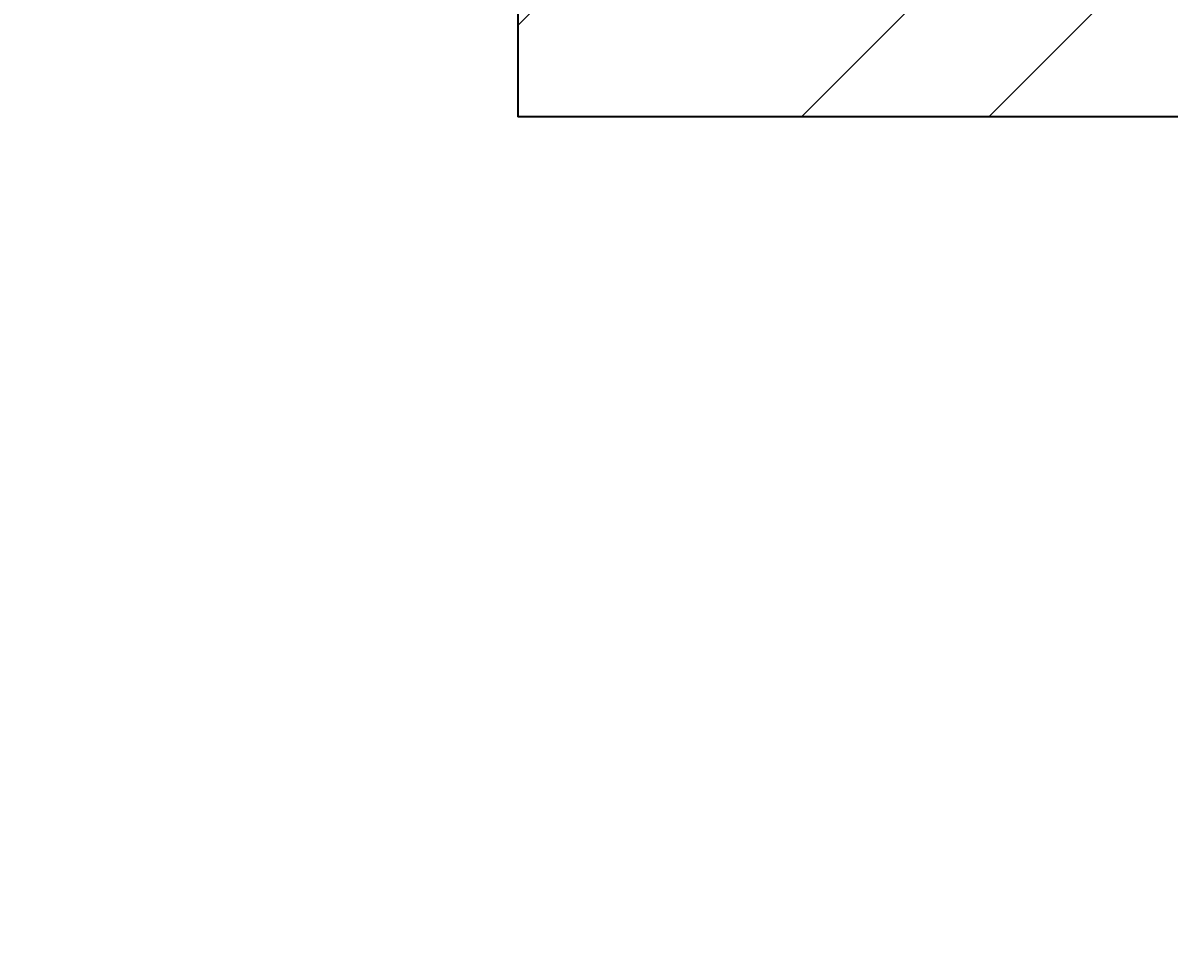
# Model space of a CAD drawing. Units: inches. Extents: x 1962 to 2771, y 1245 to 2660.
# Tile 69 of 114: x 2496 to 2523, y 2158 to 2180. Entities that reach past the tile are written whole.
import ezdxf

# ---------------------------------------------------------------- set-up
doc = ezdxf.new("R2010")
doc.units = ezdxf.units.IN
for name, color, linetype, lineweight in [('A-ANNO-DIMS', 2, 'Continuous', 18), ('A-WALL', 7, 'Continuous', 35), ('A-WALL-PATT', 252, 'Continuous', 13)]:
    doc.layers.add(name, color=color, linetype=linetype, lineweight=lineweight)
doc.styles.get("Standard").update_dxf_attribs({"font": 'arial.ttf'})
doc.dimstyles.get("Standard").update_dxf_attribs({"dimtxt": 0.18, "dimasz": 0.18, "dimexe": 0.18, "dimexo": 0.0625, "dimgap": 0.09, "dimtad": 0, "dimtih": 1, "dimtoh": 1, "dimdec": 4, "dimzin": 0, "dimdsep": 46, "dimtxsty": 'Standard', "dimcen": 0.09, "dimadec": 0, "dimazin": 0, "dimtfac": 1, "dimtdec": 4, "dimtofl": 0, "dimtmove": 0, "dimatfit": 3, "dimfxl": 1, "dimtolj": 1, "dimtzin": 0, "dimarcsym": 0})

# ---------------------------------------------------------------- blocks, each defined once
blk = doc.blocks.new('*D40')
at = {"layer": 'A-ANNO-DIMS', "color": 0, "lineweight": -2, "transparency": 16777216}
for p, q in [((2072.02, 2033.906), (2072.02, 2583.474)), ((2660.807, 2524.406), (2660.807, 2583.474)), ((2072.2, 2583.294), (2366.02, 2583.294)), ((2660.627, 2583.294), (2366.808, 2583.294))]:
    blk.add_line(p, q, dxfattribs=at)
at = {"layer": 'A-ANNO-DIMS', "color": 0, "transparency": 16777216}
for points in [[(2072.2, 2583.324), (2072.2, 2583.264), (2072.02, 2583.294)], [(2660.627, 2583.324), (2660.627, 2583.264), (2660.807, 2583.294)]]:
    blk.add_solid(points, dxfattribs=at)
at = {"layer": 'Defpoints', "color": 0, "transparency": 16777216}
for p in [(2660.807, 2583.294), (2660.807, 2524.344), (2072.02, 2033.844)]:
    blk.add_point(p, dxfattribs=at)
at = {"layer": 'A-ANNO-DIMS', "color": 0, "transparency": 16777216, "insert": (2366.414, 2583.294), "char_height": 0.18, "attachment_point": 5}
blk.add_mtext('\\A1;588.8', dxfattribs=at)

msp = doc.modelspace()

# ---------------------------------------------------------------- hatches: boundary and pattern name
at = {"layer": 'A-WALL-PATT'}
h = msp.add_hatch(dxfattribs=at)
h.set_pattern_fill('ANSI32', color=256)
h.paths.add_polyline_path([(2090.8074, 2467.3437), (2141.6481, 2467.3437), (2141.6481, 2469.5937), (2141.6481, 2471.8437), (2086.3074, 2471.8437), (2086.3074, 2422.5333), (2090.8074, 2422.5333)])
h.paths.add_polyline_path([(2282.7664, 2471.8437), (2204.8982, 2471.8437), (2204.8982, 2467.3437), (2234.8074, 2467.3437), (2234.8074, 2311.3437), (2228.7492, 2311.3437), (2228.7492, 2306.8437), (2234.8074, 2306.8437), (2331.9227, 2306.8437), (2331.9227, 2309.0937), (2331.9227, 2311.3437), (2239.3074, 2311.3437), (2239.3074, 2467.3437), (2282.7664, 2467.3437), (2282.7664, 2469.5937)])
h.paths.add_polyline_path([(2471.4531, 2519.8437), (2552.011, 2519.8437), (2564.3996, 2519.8437), (2564.3996, 2511.1389), (2568.8996, 2511.1389), (2568.8996, 2524.3437), (2466.9531, 2524.3437), (2466.9531, 2471.8437), (2450.0749, 2471.8437), (2446.4672, 2471.8437), (2446.4672, 2467.3437), (2450.0749, 2467.3437), (2475.9988, 2467.3437), (2475.9988, 2469.5937), (2475.9988, 2471.8437), (2471.4531, 2471.8437)])
h.paths.add_polyline_path([(2575.2231, 2469.5937), (2575.2231, 2471.8437), (2568.8996, 2471.8437), (2568.8996, 2487.1389), (2564.3996, 2487.1389), (2564.3996, 2471.8437), (2556.511, 2471.8437), (2499.2904, 2471.8437), (2499.2904, 2467.3437), (2507.8074, 2467.3437), (2507.8074, 2311.3437), (2414.863, 2311.3437), (2414.863, 2306.8437), (2512.3074, 2306.8437), (2517.0114, 2306.8437), (2517.0114, 2309.0937), (2517.0114, 2311.3437), (2512.3074, 2311.3437), (2512.3074, 2467.3437), (2575.2231, 2467.3437)])
h.paths.add_polyline_path([(2660.8074, 2471.8437), (2600.9602, 2471.8437), (2600.9602, 2467.3437), (2656.3074, 2467.3437), (2656.3074, 2432.5704), (2660.8074, 2432.5704)])
h.paths.add_polyline_path([(2660.8074, 2372.5704), (2656.3074, 2372.5704), (2656.3074, 2311.3437), (2600.276, 2311.3437), (2600.276, 2309.0937), (2600.276, 2306.8437), (2656.3074, 2306.8437), (2656.3074, 2296.2593), (2660.8074, 2296.2593)])
h.paths.add_polyline_path([(2572.3074, 2306.8437), (2577.1385, 2306.8437), (2577.1385, 2311.3437), (2551.082, 2311.3437), (2551.082, 2306.8437), (2567.8074, 2306.8437), (2567.8074, 2258.8437), (2540.0574, 2258.8437), (2540.0574, 2256.5937), (2540.0574, 2254.3437), (2567.8074, 2254.3437), (2656.3074, 2254.3437), (2656.3074, 2236.9085), (2660.8074, 2236.9085), (2660.8074, 2272.2593), (2656.3074, 2272.2593), (2656.3074, 2258.8437), (2572.3074, 2258.8437)])
h.paths.add_polyline_path([(2512.3074, 2254.3437), (2518.8716, 2254.3437), (2518.8716, 2256.5937), (2518.8716, 2258.8437), (2507.8074, 2258.8437), (2507.8074, 2177.8437), (2567.8074, 2177.8437), (2567.8074, 2172.9628), (2572.3074, 2172.9628), (2572.3074, 2177.8437), (2656.3074, 2177.8437), (2656.3074, 2166.4846), (2660.8074, 2166.4846), (2660.8074, 2200.9085), (2656.3074, 2200.9085), (2656.3074, 2182.3437), (2512.3074, 2182.3437)])
h.paths.add_polyline_path([(2656.3074, 2129.8437), (2572.3074, 2129.8437), (2572.3074, 2150.3044), (2570.0574, 2150.3044), (2567.8074, 2150.3044), (2567.8074, 2129.8437), (2507.8074, 2129.8437), (2507.8074, 2116.3027), (2510.0574, 2116.3027), (2512.3074, 2116.3027), (2512.3074, 2125.3437), (2567.8074, 2125.3437), (2572.3074, 2125.3437), (2656.3074, 2125.3437)])
h.paths.add_polyline_path([(2090.8074, 2362.5333), (2086.3074, 2362.5333), (2086.3074, 2298.6242), (2090.8074, 2298.6242), (2090.8074, 2306.8437), (2174.8074, 2306.8437), (2174.8074, 2286.4178), (2179.3074, 2286.4178), (2179.3074, 2306.8437), (2192.8641, 2306.8437), (2192.8641, 2309.0937), (2192.8641, 2311.3437), (2090.8074, 2311.3437)])
h.paths.add_polyline_path([(2209.156, 2258.8437), (2179.3074, 2258.8437), (2179.3074, 2263.2236), (2177.0574, 2263.2236), (2174.8074, 2263.2236), (2174.8074, 2258.8437), (2090.8074, 2258.8437), (2090.8074, 2274.6242), (2086.3074, 2274.6242), (2086.3074, 2238.2967), (2088.5574, 2238.2967), (2090.8074, 2238.2967), (2090.8074, 2254.3437), (2209.156, 2254.3437)])
h.paths.add_polyline_path([(2090.8074, 2177.8437), (2234.8074, 2177.8437), (2234.8074, 2173.1428), (2239.3074, 2173.1428), (2239.3074, 2258.8437), (2230.8442, 2258.8437), (2230.8442, 2256.5937), (2230.8442, 2254.3437), (2234.8074, 2254.3437), (2234.8074, 2182.3437), (2090.8074, 2182.3437), (2090.8074, 2202.2967), (2086.3074, 2202.2967), (2086.3074, 2140.0389), (2090.8074, 2140.0389)])
h.paths.add_polyline_path([(2090.8074, 2080.0389), (2086.3074, 2080.0389), (2086.3074, 2033.8437), (2090.8074, 2033.8437)], flags=17)
h.paths.add_polyline_path([(2244.9405, 2033.8437), (2239.3074, 2033.8437), (2239.3074, 2142.0665), (2237.2592, 2142.0665), (2234.8074, 2142.0665), (2234.8074, 2033.8437), (2090.8074, 2033.8437), (2076.5204, 2033.8437), (2072.0204, 2033.8437), (2072.0204, 2000.4493), (2076.5204, 2000.4493), (2076.5204, 2029.3437), (2090.8074, 2029.3437), (2244.9405, 2029.3437), (2244.9405, 2031.5937)])
h.paths.add_polyline_path([(2234.8074, 1933.3437), (2076.5204, 1933.3437), (2076.5204, 1952.4493), (2074.2704, 1952.4493), (2072.0204, 1952.4493), (2072.0204, 1933.3437), (2072.0204, 1928.8437), (2234.8074, 1928.8437)])
h.paths.add_polyline_path([(2090.8074, 1928.8437), (2086.3074, 1928.8437), (2086.3074, 1906.5013), (2090.8074, 1906.5013)])
h.paths.add_polyline_path([(2090.8074, 1846.5013), (2086.3074, 1846.5013), (2086.3074, 1769.9917), (2088.5574, 1769.9917), (2090.8074, 1769.9917), (2090.8074, 1780.3437), (2234.8074, 1780.3437), (2234.8074, 1708.3437), (2230.3764, 1708.3437), (2230.3764, 1703.8437), (2239.3074, 1703.8437), (2239.3074, 1792.6669), (2237.0574, 1792.6669), (2234.8074, 1792.6669), (2234.8074, 1784.8437), (2090.8074, 1784.8437)])
h.paths.add_polyline_path([(2239.3074, 1928.8437), (2244.9405, 1928.8437), (2244.9405, 1931.0937), (2244.9405, 1933.3437), (2234.8074, 1933.3437), (2234.8074, 1928.8437), (2234.8074, 1825.5949), (2239.3074, 1825.5949)])
h.paths.add_polyline_path([(2148.0425, 1649.0937), (2148.0425, 1651.3437), (2090.8074, 1651.3437), (2090.8074, 1646.8437), (2148.0425, 1646.8437)], flags=0)
h.paths.add_polyline_path([(2207.5601, 1708.3437), (2090.8074, 1708.3437), (2090.8074, 1703.8437), (2174.8074, 1703.8437), (2174.8074, 1651.3437), (2170.4457, 1651.3437), (2170.4457, 1646.8437), (2195.9924, 1646.8437), (2195.9924, 1649.0937), (2195.9924, 1651.3437), (2179.3074, 1651.3437), (2179.3074, 1703.8437), (2207.5601, 1703.8437), (2207.5601, 1706.0937)])
h.paths.add_polyline_path([(2090.8074, 1733.9917), (2086.3074, 1733.9917), (2086.3074, 1696.1032), (2088.5574, 1696.1032), (2090.8074, 1696.1032)])
h.paths.add_polyline_path([(2090.8074, 1672.1032), (2086.3074, 1672.1032), (2086.3074, 1600.3335), (2090.8074, 1600.3335)])
h.paths.add_polyline_path([(2090.8074, 1540.3335), (2086.3074, 1540.3335), (2086.3074, 1486.3437), (2139.6766, 1486.3437), (2139.6766, 1490.8437), (2090.8074, 1490.8437)])
h.paths.add_polyline_path([(2302.3876, 1490.8437), (2239.3074, 1490.8437), (2239.3074, 1646.8437), (2335.9994, 1646.8437), (2335.9994, 1651.3437), (2229.884, 1651.3437), (2229.884, 1646.8437), (2234.8074, 1646.8437), (2234.8074, 1490.8437), (2202.7103, 1490.8437), (2202.7103, 1488.5937), (2202.7103, 1486.3437), (2275.0699, 1486.3437), (2275.0699, 1475.772), (2279.5699, 1475.772), (2279.5699, 1486.3437), (2302.3876, 1486.3437)])
h.paths.add_polyline_path([(2279.5699, 1451.772), (2275.0699, 1451.772), (2275.0699, 1438.3437), (2174.8074, 1438.3437), (2174.8074, 1486.3437), (2179.7922, 1486.3437), (2179.7922, 1490.8437), (2163.3585, 1490.8437), (2163.3585, 1488.5937), (2163.3585, 1486.3437), (2170.3074, 1486.3437), (2170.3074, 1433.8437), (2279.5699, 1433.8437)])
h.paths.add_polyline_path([(2427.2363, 1490.8437), (2375.8074, 1490.8437), (2375.8074, 1646.8437), (2381.6401, 1646.8437), (2381.6401, 1651.3437), (2365.887, 1651.3437), (2365.887, 1649.0937), (2365.887, 1646.8437), (2371.3074, 1646.8437), (2371.3074, 1490.8437), (2327.5627, 1490.8437), (2327.5627, 1488.5937), (2327.5627, 1486.3437), (2371.3074, 1486.3437), (2371.3074, 1433.8437), (2375.8074, 1433.8437), (2375.8074, 1486.3437), (2427.2363, 1486.3437)])
h.paths.add_polyline_path([(2512.3074, 1646.8437), (2519.4351, 1646.8437), (2519.4351, 1649.0937), (2519.4351, 1651.3437), (2507.8074, 1651.3437), (2416.0063, 1651.3437), (2416.0063, 1649.0937), (2416.0063, 1646.8437), (2507.8074, 1646.8437), (2507.8074, 1490.8437), (2497.0532, 1490.8437), (2497.0532, 1488.5937), (2497.0532, 1486.3437), (2574.9344, 1486.3437), (2574.9344, 1476.0181), (2579.4344, 1476.0181), (2579.4344, 1486.3437), (2584.4872, 1486.3437), (2584.3074, 1490.8437), (2512.3074, 1490.8437)])
h.paths.add_polyline_path([(2470.5091, 1486.3437), (2473.9767, 1486.3437), (2473.9767, 1490.8437), (2449.6605, 1490.8437), (2449.6605, 1488.5937), (2449.6605, 1486.3437), (2466.0091, 1486.3437), (2466.0091, 1433.8437), (2470.5091, 1433.8437), (2579.4344, 1433.8437), (2579.4344, 1452.0181), (2574.9344, 1452.0181), (2574.9344, 1438.3437), (2554.5091, 1438.3437), (2470.5091, 1438.3437)])
h.paths.add_polyline_path([(2656.3074, 1490.8437), (2611.86, 1490.8437), (2611.86, 1486.3437), (2656.3074, 1486.3437)])
h.paths.add_polyline_path([(2660.8074, 1532.7007), (2658.5574, 1532.7007), (2656.3074, 1532.7007), (2656.3074, 1486.3437), (2660.8074, 1486.3437)])
h.paths.add_polyline_path([(2660.8074, 1664.9663), (2656.3074, 1664.9663), (2656.3074, 1651.3437), (2602.2313, 1651.3437), (2602.2313, 1646.8437), (2656.3074, 1646.8437), (2656.3074, 1592.7007), (2660.8074, 1592.7007)])
h.paths.add_polyline_path([(2660.8074, 1724.5221), (2656.3074, 1724.5221), (2656.3074, 1703.8437), (2542.4725, 1703.8437), (2542.4725, 1699.3437), (2567.8074, 1699.3437), (2567.8074, 1651.3437), (2552.7766, 1651.3437), (2552.7766, 1649.0937), (2552.7766, 1646.8437), (2577.2878, 1646.8437), (2577.2878, 1649.0937), (2577.2878, 1651.3437), (2572.3074, 1651.3437), (2572.3074, 1699.3437), (2656.3074, 1699.3437), (2656.3074, 1688.9663), (2660.8074, 1688.9663)])
h.paths.add_polyline_path([(2660.8074, 1880.6524), (2656.3074, 1880.6524), (2656.3074, 1832.8437), (2512.3074, 1832.8437), (2512.3074, 1837.8959), (2507.8074, 1837.8959), (2507.8074, 1828.3437), (2567.8074, 1828.3437), (2567.8074, 1804.3437), (2572.3074, 1804.3437), (2572.3074, 1828.3437), (2656.3074, 1828.3437), (2656.3074, 1818.6778), (2660.8074, 1818.6778)])
h.paths.add_polyline_path([(2660.8074, 1794.6778), (2656.3074, 1794.6778), (2656.3074, 1780.3437), (2572.3074, 1780.3437), (2572.3074, 1783.0303), (2570.0574, 1783.0303), (2567.8074, 1783.0303), (2567.8074, 1780.3437), (2507.8074, 1780.3437), (2507.8074, 1699.3437), (2517.8858, 1699.3437), (2517.8858, 1701.5937), (2517.8858, 1703.8437), (2512.3074, 1703.8437), (2512.3074, 1775.8437), (2656.3074, 1775.8437), (2656.3074, 1760.5221), (2660.8074, 1760.5221)])
h.paths.add_polyline_path([(2660.8074, 1981.3437), (2660.8074, 2020.2808), (2658.5574, 2020.2808), (2656.3074, 2020.2808), (2656.3074, 1981.3437), (2512.3074, 1981.3437), (2512.3074, 2086.6996), (2507.8074, 2086.6996), (2507.8074, 1981.3437), (2375.8074, 1981.3437), (2375.8074, 1986.8505), (2373.5574, 1986.8505), (2371.3074, 1986.8505), (2371.3074, 1973.2607), (2375.8074, 1973.2607), (2375.8074, 1976.8437), (2507.8074, 1976.8437), (2507.8074, 1865.4281), (2510.0574, 1865.4281), (2512.3074, 1865.4281), (2512.3074, 1976.8437), (2660.8074, 1976.8437)])
h.paths.add_polyline_path([(2375.8074, 1940.297), (2373.5574, 1940.297), (2371.3074, 1940.297), (2371.3074, 1933.3437), (2278.4434, 1933.3437), (2278.4434, 1928.8437), (2371.3074, 1928.8437), (2371.3074, 1651.3437), (2375.8074, 1651.3437)])
h.paths.add_polyline_path([(2660.8074, 1976.8437), (2656.3074, 1976.8437), (2656.3074, 1940.6524), (2660.8074, 1940.6524)], flags=17)
h.paths.add_polyline_path([(2660.8074, 2142.4846), (2656.3074, 2142.4846), (2656.3074, 2080.2808), (2660.8074, 2080.2808)])
h.paths.add_polyline_path([(2381.4189, 2311.3437), (2375.8074, 2311.3437), (2375.8074, 2467.3437), (2424.7242, 2467.3437), (2424.7242, 2469.5937), (2424.7242, 2471.8437), (2375.8074, 2471.8437), (2375.8074, 2524.3437), (2371.3074, 2524.3437), (2371.3074, 2471.8437), (2307.2097, 2471.8437), (2307.2097, 2467.3437), (2371.3074, 2467.3437), (2371.3074, 2311.3437), (2366.8901, 2311.3437), (2366.8901, 2306.8437), (2371.3074, 2306.8437), (2371.3074, 2033.8437), (2279.6589, 2033.8437), (2279.6589, 2029.3437), (2371.3074, 2029.3437), (2371.3074, 2014.2598), (2375.8074, 2014.2598), (2375.8074, 2306.8437), (2381.4189, 2306.8437)])
h.paths.add_polyline_path([(2263.3074, 2524.3437), (2170.3074, 2524.3437), (2170.3074, 2519.8437), (2170.3074, 2471.8437), (2165.0312, 2471.8437), (2165.0312, 2467.3437), (2179.6721, 2467.3437), (2179.6721, 2469.5161), (2179.6721, 2471.8437), (2174.8074, 2471.8437), (2174.8074, 2519.8437), (2258.8074, 2519.8437), (2258.8074, 2511.6436), (2263.3074, 2511.6436)])
h.paths.add_polyline_path([(2245.0232, 1361.4123), (2492.9468, 1361.4123), (2492.9468, 1398.505), (2245.0232, 1398.505)], flags=9)
h.paths.add_polyline_path([(2388.1434, 2086.6936), (2425.0704, 2086.6936), (2425.0704, 2105.3509), (2388.1434, 2105.3509)], flags=9)
h.paths.add_polyline_path([(2404.922, 2242.6744), (2445.7337, 2242.6744), (2445.7337, 2261.3318), (2404.922, 2261.3318)], flags=9)
h.paths.add_polyline_path([(2269.4107, 2156.7935), (2306.3378, 2156.7935), (2306.3378, 2175.4508), (2269.4107, 2175.4508)], flags=9)
h.paths.add_polyline_path([(2269.3277, 2233.4343), (2306.2547, 2233.4343), (2306.2547, 2252.0917), (2269.3277, 2252.0917)], flags=9)
h.paths.add_polyline_path([(2431.6052, 2320.6922), (2470.4456, 2320.6922), (2470.4456, 2339.3495), (2431.6052, 2339.3495)], flags=25)
h.paths.add_polyline_path([(2249.6902, 2315.7608), (2288.5306, 2315.7608), (2288.5306, 2334.4182), (2249.6902, 2334.4182)], flags=25)
h.paths.add_polyline_path([(2096.9301, 2314.3181), (2135.7704, 2314.3181), (2135.7704, 2332.9755), (2096.9301, 2332.9755)], flags=25)
h.paths.add_polyline_path([(2134.3475, 2285.7089), (2161.4655, 2285.7089), (2161.4655, 2304.3662), (2134.3475, 2304.3662)], flags=9)
h.paths.add_polyline_path([(2126.5155, 2209.4076), (2159.9227, 2209.4076), (2159.9227, 2228.065), (2126.5155, 2228.065)], flags=25)
h.paths.add_polyline_path([(2110.5753, 2141.5299), (2149.4157, 2141.5299), (2149.4157, 2160.1872), (2110.5753, 2160.1872)], flags=25)
h.paths.add_polyline_path([(2249.8618, 1968.3317), (2286.3966, 1968.3317), (2286.3966, 1986.989), (2249.8618, 1986.989)], flags=9)
h.paths.add_polyline_path([(2395.9507, 1777.0051), (2436.7624, 1777.0051), (2436.7624, 1795.6625), (2395.9507, 1795.6625)], flags=9)
h.paths.add_polyline_path([(2398.5259, 1888.5651), (2435.0062, 1888.5651), (2435.0062, 1907.2224), (2398.5259, 1907.2224)], flags=25)
h.paths.add_polyline_path([(2259.3506, 1728.3559), (2296.2776, 1728.3559), (2296.2776, 1747.0132), (2259.3506, 1747.0132)], flags=9)
h.paths.add_polyline_path([(2271.3698, 1845.268), (2308.2968, 1845.268), (2308.2968, 1863.9253), (2271.3698, 1863.9253)], flags=9)
h.paths.add_polyline_path([(2120.9355, 1786.3027), (2159.7759, 1786.3027), (2159.7759, 1804.9601), (2120.9355, 1804.9601)], flags=25)
h.paths.add_polyline_path([(2121.3164, 1732.1043), (2154.7236, 1732.1043), (2154.7236, 1750.7616), (2121.3164, 1750.7616)], flags=25)
h.paths.add_polyline_path([(2118.3706, 1678.8997), (2147.5282, 1678.8997), (2147.5282, 1697.557), (2118.3706, 1697.557)], flags=25)
h.paths.add_polyline_path([(2385.9227, 1493.557), (2424.763, 1493.557), (2424.763, 1512.2143), (2385.9227, 1512.2143)], flags=25)
h.paths.add_polyline_path([(2248.7058, 1500.0256), (2287.5462, 1500.0256), (2287.5462, 1518.6829), (2248.7058, 1518.6829)], flags=25)
h.paths.add_polyline_path([(2104.1669, 1617.3771), (2143.0073, 1617.3771), (2143.0073, 1636.0344), (2104.1669, 1636.0344)], flags=9)
h.paths.add_polyline_path([(2096.0714, 1447.8824), (2137.3845, 1447.8824), (2137.3845, 1458.1859), (2096.0714, 1458.1859)], flags=9)
h.paths.add_polyline_path([(2180.6114, 1440.325), (2209.7689, 1440.325), (2209.7689, 1458.9823), (2180.6114, 1458.9823)], flags=25)
h.paths.add_polyline_path([(2316.1698, 1447.9637), (2357.4829, 1447.9637), (2357.4829, 1458.2673), (2316.1698, 1458.2673)], flags=9)
h.paths.add_polyline_path([(2397.6187, 1447.9637), (2438.9318, 1447.9637), (2438.9318, 1458.2673), (2397.6187, 1458.2673)], flags=9)
h.paths.add_polyline_path([(2473.0778, 1439.5953), (2502.2354, 1439.5953), (2502.2354, 1458.2527), (2473.0778, 1458.2527)], flags=25)
h.paths.add_polyline_path([(2589.7027, 1447.8819), (2631.0158, 1447.8819), (2631.0158, 1458.1855), (2589.7027, 1458.1855)], flags=9)
h.paths.add_polyline_path([(2522.4009, 1497.5285), (2561.2413, 1497.5285), (2561.2413, 1516.1859), (2522.4009, 1516.1859)], flags=25)
h.paths.add_polyline_path([(2579.6565, 1671.3482), (2608.8141, 1671.3482), (2608.8141, 1690.0056), (2579.6565, 1690.0056)], flags=25)
h.paths.add_polyline_path([(2544.7038, 1725.5064), (2578.1111, 1725.5064), (2578.1111, 1744.1637), (2544.7038, 1744.1637)], flags=25)
h.paths.add_polyline_path([(2578.1191, 1807.472), (2607.2766, 1807.472), (2607.2766, 1826.1293), (2578.1191, 1826.1293)], flags=25)
h.paths.add_polyline_path([(2595.0614, 1835.1839), (2633.9018, 1835.1839), (2633.9018, 1853.8413), (2595.0614, 1853.8413)], flags=25)
h.paths.add_polyline_path([(2567.0097, 2097.7035), (2605.8501, 2097.7035), (2605.8501, 2116.3609), (2567.0097, 2116.3609)], flags=9)
h.paths.add_polyline_path([(2586.644, 2134.6454), (2615.8015, 2134.6454), (2615.8015, 2153.3027), (2586.644, 2153.3027)], flags=9)
h.paths.add_polyline_path([(2544.6185, 2212.6783), (2578.0258, 2212.6783), (2578.0258, 2231.3356), (2544.6185, 2231.3356)], flags=25)
h.paths.add_polyline_path([(2577.0273, 2256.9023), (2606.1849, 2256.9023), (2606.1849, 2275.5597), (2577.0273, 2275.5597)], flags=24)
h.paths.add_polyline_path([(2605.2683, 2315.2821), (2644.1087, 2315.2821), (2644.1087, 2333.9395), (2605.2683, 2333.9395)], flags=25)
h.paths.add_polyline_path([(2583.1244, 2496.1815), (2624.4375, 2496.1815), (2624.4375, 2506.4851), (2583.1244, 2506.4851)], flags=9)
h.paths.add_polyline_path([(2474.761, 2497.0823), (2503.9185, 2497.0823), (2503.9185, 2515.7397), (2474.761, 2515.7397)], flags=25)
h.paths.add_polyline_path([(2387.5787, 2494.2563), (2428.902, 2494.2563), (2428.902, 2504.5598), (2387.5787, 2504.5598)], flags=9)
h.paths.add_polyline_path([(2300.1657, 2500.1564), (2341.4788, 2500.1564), (2341.4788, 2510.46), (2300.1657, 2510.46)], flags=25)
h.paths.add_polyline_path([(2176.8589, 2497.5843), (2206.0165, 2497.5843), (2206.0165, 2516.2416), (2176.8589, 2516.2416)], flags=25)
h.paths.add_polyline_path([(2097.4668, 2494.9762), (2138.7799, 2494.9762), (2138.7799, 2505.2798), (2097.4668, 2505.2798)], flags=9)

# ---------------------------------------------------------------- linework, layer by layer
at = {"layer": 'A-WALL'}
for p in [(2507.8074, 2258.8437), (2567.8074, 2177.8437)]:
    msp.add_line(p, (2507.8074, 2177.8437), dxfattribs=at)

# ---------------------------------------------------------------- dimensions: what is measured, and where the dimension line sits
at = {"layer": 'A-ANNO-DIMS'}
dim = msp.add_linear_dim(base=(2660.8074, 2583.2937), p1=(2072.0204, 2033.8437), p2=(2660.8074, 2524.3437), dimstyle='Standard', override={"dimdec": 1, "dimlfac": 1, "dimrnd": 0, "dimzin": 0, "dimdsep": 46, "dimlunit": 2}, dxfattribs=at)
dim.commit()
dim.dimension.update_dxf_attribs({"geometry": '*D40', "text_midpoint": (2366.4139, 2583.2937)})

doc.saveas('drawing.dxf')
